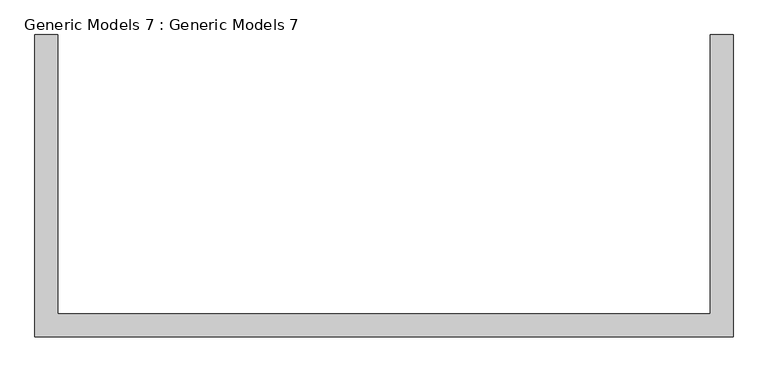
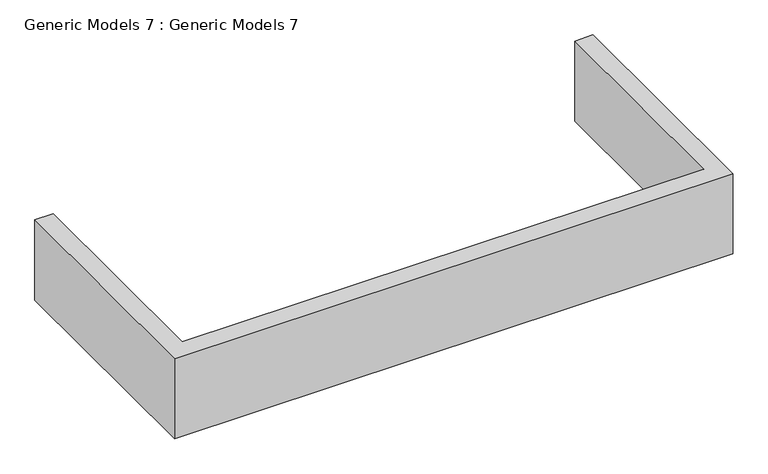
"""IFC4 building model written with IfcOpenShell, lengths in millimetres: proxy geometry, Generic Models 7 : Generic Models 7."""

from ifc_helpers import new_model, si_unit, frame, origin, place, context, project, spatial, polyline, outline, extrude, source, transform, mapped, element, save


def generic_models_7_generic_models_7_ebfadceb(model_context):
    return source(origin(), model_context, "Body", "SweptSolid", [
        extrude(outline(polyline([(-4771.7270642, -10271.3896616), (-4644.7270642, -10271.3896616), (-4644.7270642, -11812.34549), (-1047.1658472, -11812.34549), (-1047.1658472, -10271.3896616), (-920.1658472, -10271.3896616), (-920.1658472, -11939.34549), (-4771.7270642, -11939.34549), (-4771.7270642, -10271.3896616)])), frame((0.0, 0.0, 2768.6), z_axis=(0.0, 0.0, 1.0), x_axis=(1.0, 0.0, 0.0)), (0.0, 0.0, 1.0), 584.2),
    ])


if __name__ == "__main__":
    model = new_model("IFC4")
    model_context = context("Model", 3, world=origin())
    ifc_project = project(units=[si_unit("LENGTHUNIT", "METRE", prefix="MILLI")], contexts=[model_context])
    site = spatial("IfcSite", under=ifc_project)
    building = spatial("IfcBuilding", under=site)
    placement = place(None, origin())
    generic_models_7_generic_models_7_shape = generic_models_7_generic_models_7_ebfadceb(model_context)
    element("IfcBuildingElementProxy", 1, Name="Generic Models 7 : Generic Models 7", ObjectType="Generic Models 7 : Generic Models 7", at=placement, inside=building, context=model_context, shape_type="MappedRepresentation", body=[
        mapped(generic_models_7_generic_models_7_shape, transform((0.0, 0.0, 0.0), x_axis=(1.0, 0.0, 0.0), y_axis=(0.0, 1.0, 0.0), z_axis=(0.0, 0.0, 1.0))),
    ])
    save(model, "model.ifc")

# Revit data of these elements
# Element 1 (IfcBuildingElementProxy, "Generic Models 7 : Generic Models 7")
#   Materials on its faces: "white colour"
# Materials
#   "white colour": class "Generic", colour RGB 120 120 120, transparency 0, Cost = 0
